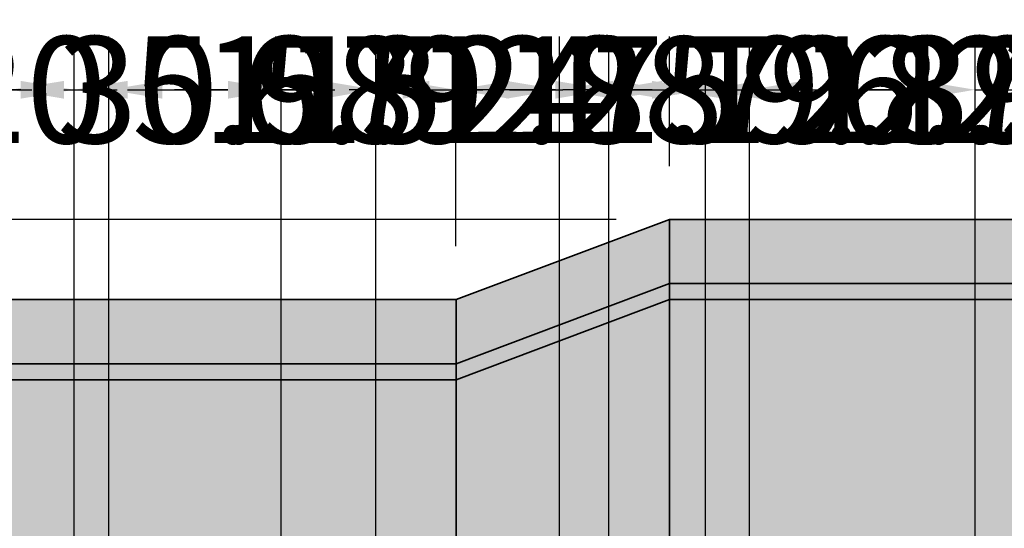
# Model space of a CAD drawing. Units: millimetres. Extents: x 130 to 1021, y 147 to 699.
# Tile 35 of 40: x 366 to 550, y 604 to 699. Entities that reach past the tile are written whole.
import ezdxf

# ---------------------------------------------------------------- set-up
doc = ezdxf.new("R2010")
doc.units = ezdxf.units.MM
doc.header["$MEASUREMENT"] = 0
for name, color, linetype, lineweight in [('A-ANNO-DIMS', 2, 'Continuous', 18), ('A-ELEV', 7, 'Continuous', 35), ('A-ELEV-PATT', 9, 'Continuous', 13)]:
    doc.layers.add(name, color=color, linetype=linetype, lineweight=lineweight)
doc.styles.get("Standard").update_dxf_attribs({"font": 'arial.ttf'})
doc.dimstyles.get("Standard").update_dxf_attribs({"dimtxt": 20, "dimasz": 10, "dimexe": 10, "dimexo": 10, "dimgap": 5, "dimtad": 0, "dimtih": 1, "dimtoh": 1, "dimdec": 0, "dimzin": 0, "dimdsep": 46, "dimtxsty": 'Standard', "dimcen": 5, "dimadec": 0, "dimazin": 0, "dimtfac": 1, "dimtdec": 0, "dimtofl": 0, "dimtmove": 0, "dimatfit": 3, "dimfxl": 1, "dimtolj": 1, "dimtzin": 0, "dimarcsym": 0})

# ---------------------------------------------------------------- blocks, each defined once
blk = doc.blocks.new('*D11')
at = {"layer": 'A-ANNO-DIMS', "color": 0, "lineweight": -2, "transparency": 16777216}
for p, q in [((737.37, 648.7), (737.37, 149.74)), ((299.37, 566.95), (299.37, 149.74)), ((309.37, 159.74), (490.86, 159.74)), ((727.37, 159.74), (545.89, 159.74))]:
    blk.add_line(p, q, dxfattribs=at)
at = {"layer": 'A-ANNO-DIMS', "color": 0, "transparency": 16777216}
for points in [[(309.37, 161.41), (309.37, 158.07), (299.37, 159.74)], [(727.37, 161.41), (727.37, 158.07), (737.37, 159.74)]]:
    blk.add_solid(points, dxfattribs=at)
at = {"layer": 'Defpoints', "color": 0, "transparency": 16777216}
for p in [(737.37, 658.7), (299.37, 576.95), (737.37, 159.74)]:
    blk.add_point(p, dxfattribs=at)
at = {"layer": 'A-ANNO-DIMS', "color": 0, "transparency": 16777216, "insert": (518.37, 159.74), "char_height": 20, "attachment_point": 5}
blk.add_mtext('\\A1;438', dxfattribs=at)
blk = doc.blocks.new('*D12')
at = {"layer": 'A-ANNO-DIMS', "color": 0, "lineweight": -2, "transparency": 16777216}
for p, q in [((477.37, 661.95), (265.07, 661.95)), ((275.07, 651.95), (275.07, 438.2)), ((275.07, 194.04), (275.07, 407.78)), ((357.16, 184.04), (265.07, 184.04))]:
    blk.add_line(p, q, dxfattribs=at)
at = {"layer": 'A-ANNO-DIMS', "color": 0, "transparency": 16777216}
for points in [[(273.41, 651.95), (276.74, 651.95), (275.07, 661.95)], [(273.41, 194.04), (276.74, 194.04), (275.07, 184.04)]]:
    blk.add_solid(points, dxfattribs=at)
at = {"layer": 'Defpoints', "color": 0, "transparency": 16777216}
for p in [(275.07, 661.95), (487.37, 661.95), (367.16, 184.04)]:
    blk.add_point(p, dxfattribs=at)
at = {"layer": 'A-ANNO-DIMS', "color": 0, "transparency": 16777216, "insert": (275.07, 422.99), "char_height": 20, "attachment_point": 5}
blk.add_mtext('\\A1;477.9', dxfattribs=at)
blk = doc.blocks.new('*D14')
at = {"layer": 'A-ANNO-DIMS', "color": 0, "lineweight": -2, "transparency": 16777216}
for p, q in [((307.37, 641.95), (307.37, 696.25)), ((327.37, 579.88), (327.37, 696.25)), ((297.37, 686.25), (287.37, 686.25)), ((337.37, 686.25), (347.37, 686.25))]:
    blk.add_line(p, q, dxfattribs=at)
at = {"layer": 'A-ANNO-DIMS', "color": 0, "transparency": 16777216}
for points in [[(297.37, 687.91), (297.37, 684.58), (307.37, 686.25)], [(337.37, 687.91), (337.37, 684.58), (327.37, 686.25)]]:
    blk.add_solid(points, dxfattribs=at)
at = {"layer": 'Defpoints', "color": 0, "transparency": 16777216}
for p in [(327.37, 686.25), (307.37, 631.95), (327.37, 569.88)]:
    blk.add_point(p, dxfattribs=at)
at = {"layer": 'A-ANNO-DIMS', "color": 0, "transparency": 16777216, "insert": (366.83, 686.25), "char_height": 20, "attachment_point": 5}
blk.add_mtext('\\A1;20', dxfattribs=at)
blk = doc.blocks.new('*D15')
at = {"layer": 'A-ANNO-DIMS', "color": 0, "lineweight": -2, "transparency": 16777216}
for p, q in [((327.37, 579.88), (327.37, 696.25)), ((357.94, 411.95), (357.94, 696.25)), ((337.37, 686.25), (347.94, 686.25)), ((357.94, 686.25), (367.94, 686.25))]:
    blk.add_line(p, q, dxfattribs=at)
at = {"layer": 'A-ANNO-DIMS', "color": 0, "transparency": 16777216}
for points in [[(337.37, 687.91), (337.37, 684.58), (327.37, 686.25)], [(347.94, 687.91), (347.94, 684.58), (357.94, 686.25)]]:
    blk.add_solid(points, dxfattribs=at)
at = {"layer": 'Defpoints', "color": 0, "transparency": 16777216}
for p in [(357.94, 686.25), (327.37, 569.88), (357.94, 401.95)]:
    blk.add_point(p, dxfattribs=at)
at = {"layer": 'A-ANNO-DIMS', "color": 0, "transparency": 16777216, "insert": (406.68, 686.25), "char_height": 20, "attachment_point": 5}
blk.add_mtext('\\A1;30.57', dxfattribs=at)
blk = doc.blocks.new('*D16')
at = {"layer": 'A-ANNO-DIMS', "color": 0, "lineweight": -2, "transparency": 16777216}
for p, q in [((357.94, 411.95), (357.94, 696.25)), ((363.92, 579.88), (363.92, 696.25)), ((347.94, 686.25), (337.94, 686.25)), ((373.92, 686.25), (383.92, 686.25))]:
    blk.add_line(p, q, dxfattribs=at)
at = {"layer": 'A-ANNO-DIMS', "color": 0, "transparency": 16777216}
for points in [[(347.94, 687.91), (347.94, 684.58), (357.94, 686.25)], [(373.92, 687.91), (373.92, 684.58), (363.92, 686.25)]]:
    blk.add_solid(points, dxfattribs=at)
at = {"layer": 'Defpoints', "color": 0, "transparency": 16777216}
for p in [(363.92, 686.25), (363.92, 569.88), (357.94, 401.95)]:
    blk.add_point(p, dxfattribs=at)
at = {"layer": 'A-ANNO-DIMS', "color": 0, "transparency": 16777216, "insert": (420.74, 686.25), "char_height": 20, "attachment_point": 5}
blk.add_mtext('\\A1;5.981', dxfattribs=at)
blk = doc.blocks.new('*D17')
at = {"layer": 'A-ANNO-DIMS', "color": 0, "lineweight": -2, "transparency": 16777216}
for p, q in [((363.92, 579.88), (363.92, 696.25)), ((375.85, 490.22), (375.85, 696.25)), ((353.92, 686.25), (343.92, 686.25)), ((385.85, 686.25), (395.85, 686.25))]:
    blk.add_line(p, q, dxfattribs=at)
at = {"layer": 'A-ANNO-DIMS', "color": 0, "transparency": 16777216}
for points in [[(353.92, 687.91), (353.92, 684.58), (363.92, 686.25)], [(385.85, 687.91), (385.85, 684.58), (375.85, 686.25)]]:
    blk.add_solid(points, dxfattribs=at)
at = {"layer": 'Defpoints', "color": 0, "transparency": 16777216}
for p in [(375.85, 686.25), (363.92, 569.88), (375.85, 480.22)]:
    blk.add_point(p, dxfattribs=at)
at = {"layer": 'A-ANNO-DIMS', "color": 0, "transparency": 16777216, "insert": (441.44, 686.25), "char_height": 20, "attachment_point": 5}
blk.add_mtext('\\A1;11.928', dxfattribs=at)
blk = doc.blocks.new('*D18')
at = {"layer": 'A-ANNO-DIMS', "color": 0, "lineweight": -2, "transparency": 16777216}
for p, q in [((375.85, 490.22), (375.85, 696.25)), ((382.37, 388.95), (382.37, 696.25)), ((365.85, 686.25), (355.85, 686.25)), ((392.37, 686.25), (402.37, 686.25))]:
    blk.add_line(p, q, dxfattribs=at)
at = {"layer": 'A-ANNO-DIMS', "color": 0, "transparency": 16777216}
for points in [[(365.85, 687.91), (365.85, 684.58), (375.85, 686.25)], [(392.37, 687.91), (392.37, 684.58), (382.37, 686.25)]]:
    blk.add_solid(points, dxfattribs=at)
at = {"layer": 'Defpoints', "color": 0, "transparency": 16777216}
for p in [(382.37, 686.25), (375.85, 480.22), (382.37, 378.95)]:
    blk.add_point(p, dxfattribs=at)
at = {"layer": 'A-ANNO-DIMS', "color": 0, "transparency": 16777216, "insert": (441.13, 686.25), "char_height": 20, "attachment_point": 5}
blk.add_mtext('\\A1;6.524', dxfattribs=at)
blk = doc.blocks.new('*D19')
at = {"layer": 'A-ANNO-DIMS', "color": 0, "lineweight": -2, "transparency": 16777216}
for p, q in [((382.37, 388.95), (382.37, 696.25)), ((414.65, 510.88), (414.65, 696.25)), ((392.37, 686.25), (404.65, 686.25)), ((414.65, 686.25), (424.65, 686.25))]:
    blk.add_line(p, q, dxfattribs=at)
at = {"layer": 'A-ANNO-DIMS', "color": 0, "transparency": 16777216}
for points in [[(392.37, 687.91), (392.37, 684.58), (382.37, 686.25)], [(404.65, 687.91), (404.65, 684.58), (414.65, 686.25)]]:
    blk.add_solid(points, dxfattribs=at)
at = {"layer": 'Defpoints', "color": 0, "transparency": 16777216}
for p in [(414.65, 686.25), (414.65, 500.88), (382.37, 378.95)]:
    blk.add_point(p, dxfattribs=at)
at = {"layer": 'A-ANNO-DIMS', "color": 0, "transparency": 16777216, "insert": (463.41, 686.25), "char_height": 20, "attachment_point": 5}
blk.add_mtext('\\A1;32.28', dxfattribs=at)
blk = doc.blocks.new('*D20')
at = {"layer": 'A-ANNO-DIMS', "color": 0, "lineweight": -2, "transparency": 16777216}
for p, q in [((414.65, 510.88), (414.65, 696.25)), ((432.37, 388.95), (432.37, 696.25)), ((404.65, 686.25), (394.65, 686.25)), ((442.37, 686.25), (452.37, 686.25))]:
    blk.add_line(p, q, dxfattribs=at)
at = {"layer": 'A-ANNO-DIMS', "color": 0, "transparency": 16777216}
for points in [[(404.65, 687.91), (404.65, 684.58), (414.65, 686.25)], [(442.37, 687.91), (442.37, 684.58), (432.37, 686.25)]]:
    blk.add_solid(points, dxfattribs=at)
at = {"layer": 'Defpoints', "color": 0, "transparency": 16777216}
for p in [(432.37, 686.25), (414.65, 500.88), (432.37, 378.95)]:
    blk.add_point(p, dxfattribs=at)
at = {"layer": 'A-ANNO-DIMS', "color": 0, "transparency": 16777216, "insert": (490.08, 686.25), "char_height": 20, "attachment_point": 5}
blk.add_mtext('\\A1;17.72', dxfattribs=at)
blk = doc.blocks.new('*D21')
at = {"layer": 'A-ANNO-DIMS', "color": 0, "lineweight": -2, "transparency": 16777216}
for p, q in [((432.37, 388.95), (432.37, 696.25)), ((447.37, 656.95), (447.37, 696.25)), ((422.37, 686.25), (412.37, 686.25)), ((457.37, 686.25), (467.37, 686.25))]:
    blk.add_line(p, q, dxfattribs=at)
at = {"layer": 'A-ANNO-DIMS', "color": 0, "transparency": 16777216}
for points in [[(422.37, 687.91), (422.37, 684.58), (432.37, 686.25)], [(457.37, 687.91), (457.37, 684.58), (447.37, 686.25)]]:
    blk.add_solid(points, dxfattribs=at)
at = {"layer": 'Defpoints', "color": 0, "transparency": 16777216}
for p in [(447.37, 686.25), (447.37, 646.95), (432.37, 378.95)]:
    blk.add_point(p, dxfattribs=at)
at = {"layer": 'A-ANNO-DIMS', "color": 0, "transparency": 16777216, "insert": (485.83, 686.25), "char_height": 20, "attachment_point": 5}
blk.add_mtext('\\A1;15', dxfattribs=at)
blk = doc.blocks.new('*D22')
at = {"layer": 'A-ANNO-DIMS', "color": 0, "lineweight": -2, "transparency": 16777216}
for p, q in [((447.37, 656.95), (447.37, 696.25)), ((466.77, 403.95), (466.77, 696.25)), ((437.37, 686.25), (427.37, 686.25)), ((476.77, 686.25), (486.77, 686.25))]:
    blk.add_line(p, q, dxfattribs=at)
at = {"layer": 'A-ANNO-DIMS', "color": 0, "transparency": 16777216}
for points in [[(437.37, 687.91), (437.37, 684.58), (447.37, 686.25)], [(476.77, 687.91), (476.77, 684.58), (466.77, 686.25)]]:
    blk.add_solid(points, dxfattribs=at)
at = {"layer": 'Defpoints', "color": 0, "transparency": 16777216}
for p in [(466.77, 686.25), (447.37, 646.95), (466.77, 393.95)]:
    blk.add_point(p, dxfattribs=at)
at = {"layer": 'A-ANNO-DIMS', "color": 0, "transparency": 16777216, "insert": (532.34, 686.25), "char_height": 20, "attachment_point": 5}
blk.add_mtext('\\A1;19.393', dxfattribs=at)
blk = doc.blocks.new('*D23')
at = {"layer": 'A-ANNO-DIMS', "color": 0, "lineweight": -2, "transparency": 16777216}
for p, q in [((466.77, 403.95), (466.77, 696.25)), ((475.99, 209.04), (475.99, 696.25)), ((456.77, 686.25), (446.77, 686.25)), ((485.99, 686.25), (495.99, 686.25))]:
    blk.add_line(p, q, dxfattribs=at)
at = {"layer": 'A-ANNO-DIMS', "color": 0, "transparency": 16777216}
for points in [[(456.77, 687.91), (456.77, 684.58), (466.77, 686.25)], [(485.99, 687.91), (485.99, 684.58), (475.99, 686.25)]]:
    blk.add_solid(points, dxfattribs=at)
at = {"layer": 'Defpoints', "color": 0, "transparency": 16777216}
for p in [(475.99, 686.25), (466.77, 393.95), (475.99, 199.04)]:
    blk.add_point(p, dxfattribs=at)
at = {"layer": 'A-ANNO-DIMS', "color": 0, "transparency": 16777216, "insert": (534.63, 686.25), "char_height": 20, "attachment_point": 5}
blk.add_mtext('\\A1;9.222', dxfattribs=at)
blk = doc.blocks.new('*D24')
at = {"layer": 'A-ANNO-DIMS', "color": 0, "lineweight": -2, "transparency": 16777216}
for p, q in [((475.99, 209.04), (475.99, 696.25)), ((487.37, 671.95), (487.37, 696.25)), ((465.99, 686.25), (455.99, 686.25)), ((497.37, 686.25), (507.37, 686.25))]:
    blk.add_line(p, q, dxfattribs=at)
at = {"layer": 'A-ANNO-DIMS', "color": 0, "transparency": 16777216}
for points in [[(465.99, 687.91), (465.99, 684.58), (475.99, 686.25)], [(497.37, 687.91), (497.37, 684.58), (487.37, 686.25)]]:
    blk.add_solid(points, dxfattribs=at)
at = {"layer": 'Defpoints', "color": 0, "transparency": 16777216}
for p in [(487.37, 686.25), (487.37, 661.95), (475.99, 199.04)]:
    blk.add_point(p, dxfattribs=at)
at = {"layer": 'A-ANNO-DIMS', "color": 0, "transparency": 16777216, "insert": (553.02, 686.25), "char_height": 20, "attachment_point": 5}
blk.add_mtext('\\A1;11.385', dxfattribs=at)
blk = doc.blocks.new('*D25')
at = {"layer": 'A-ANNO-DIMS', "color": 0, "lineweight": -2, "transparency": 16777216}
for p, q in [((487.37, 671.95), (487.37, 696.25)), ((494.1, 506.91), (494.1, 696.25)), ((477.37, 686.25), (467.37, 686.25)), ((504.1, 686.25), (514.1, 686.25))]:
    blk.add_line(p, q, dxfattribs=at)
at = {"layer": 'A-ANNO-DIMS', "color": 0, "transparency": 16777216}
for points in [[(477.37, 687.91), (477.37, 684.58), (487.37, 686.25)], [(504.1, 687.91), (504.1, 684.58), (494.1, 686.25)]]:
    blk.add_solid(points, dxfattribs=at)
at = {"layer": 'Defpoints', "color": 0, "transparency": 16777216}
for p in [(494.1, 686.25), (487.37, 661.95), (494.1, 496.91)]:
    blk.add_point(p, dxfattribs=at)
at = {"layer": 'A-ANNO-DIMS', "color": 0, "transparency": 16777216, "insert": (552.92, 686.25), "char_height": 20, "attachment_point": 5}
blk.add_mtext('\\A1;6.728', dxfattribs=at)
blk = doc.blocks.new('*D26')
at = {"layer": 'A-ANNO-DIMS', "color": 0, "lineweight": -2, "transparency": 16777216}
for p, q in [((494.1, 506.91), (494.1, 696.25)), ((502.37, 593.95), (502.37, 696.25)), ((484.1, 686.25), (474.1, 686.25)), ((512.37, 686.25), (522.37, 686.25))]:
    blk.add_line(p, q, dxfattribs=at)
at = {"layer": 'A-ANNO-DIMS', "color": 0, "transparency": 16777216}
for points in [[(484.1, 687.91), (484.1, 684.58), (494.1, 686.25)], [(512.37, 687.91), (512.37, 684.58), (502.37, 686.25)]]:
    blk.add_solid(points, dxfattribs=at)
at = {"layer": 'Defpoints', "color": 0, "transparency": 16777216}
for p in [(502.37, 686.25), (502.37, 583.95), (494.1, 496.91)]:
    blk.add_point(p, dxfattribs=at)
at = {"layer": 'A-ANNO-DIMS', "color": 0, "transparency": 16777216, "insert": (561.03, 686.25), "char_height": 20, "attachment_point": 5}
blk.add_mtext('\\A1;8.272', dxfattribs=at)
blk = doc.blocks.new('*D27')
at = {"layer": 'A-ANNO-DIMS', "color": 0, "lineweight": -2, "transparency": 16777216}
for p, q in [((502.37, 593.95), (502.37, 696.25)), ((544.64, 396.26), (544.64, 696.25)), ((512.37, 686.25), (534.64, 686.25)), ((544.64, 686.25), (554.64, 686.25))]:
    blk.add_line(p, q, dxfattribs=at)
at = {"layer": 'A-ANNO-DIMS', "color": 0, "transparency": 16777216}
for points in [[(512.37, 687.91), (512.37, 684.58), (502.37, 686.25)], [(534.64, 687.91), (534.64, 684.58), (544.64, 686.25)]]:
    blk.add_solid(points, dxfattribs=at)
at = {"layer": 'Defpoints', "color": 0, "transparency": 16777216}
for p in [(544.64, 686.25), (502.37, 583.95), (544.64, 386.26)]:
    blk.add_point(p, dxfattribs=at)
at = {"layer": 'A-ANNO-DIMS', "color": 0, "transparency": 16777216, "insert": (593.78, 686.25), "char_height": 20, "attachment_point": 5}
blk.add_mtext('\\A1;42.26', dxfattribs=at)
blk = doc.blocks.new('*D28')
at = {"layer": 'A-ANNO-DIMS', "color": 0, "lineweight": -2, "transparency": 16777216}
for p, q in [((544.64, 396.26), (544.64, 696.25)), ((552.37, 593.95), (552.37, 696.25)), ((534.64, 686.25), (524.64, 686.25)), ((562.37, 686.25), (572.37, 686.25))]:
    blk.add_line(p, q, dxfattribs=at)
at = {"layer": 'A-ANNO-DIMS', "color": 0, "transparency": 16777216}
for points in [[(534.64, 687.91), (534.64, 684.58), (544.64, 686.25)], [(562.37, 687.91), (562.37, 684.58), (552.37, 686.25)]]:
    blk.add_solid(points, dxfattribs=at)
at = {"layer": 'Defpoints', "color": 0, "transparency": 16777216}
for p in [(552.37, 686.25), (552.37, 583.95), (544.64, 386.26)]:
    blk.add_point(p, dxfattribs=at)
at = {"layer": 'A-ANNO-DIMS', "color": 0, "transparency": 16777216, "insert": (611.06, 686.25), "char_height": 20, "attachment_point": 5}
blk.add_mtext('\\A1;7.738', dxfattribs=at)
blk = doc.blocks.new('*D57')
at = {"layer": 'A-ANNO-DIMS', "color": 0, "lineweight": -2, "transparency": 16777216}
for p, q in [((761.67, 606.95), (761.67, 616.95)), ((761.67, 616.95), (771.67, 616.95)), ((497.37, 596.95), (771.67, 596.95)), ((562.37, 583.95), (771.67, 583.95)), ((761.67, 573.95), (761.67, 563.95))]:
    blk.add_line(p, q, dxfattribs=at)
at = {"layer": 'A-ANNO-DIMS', "color": 0, "transparency": 16777216}
for points in [[(760.01, 606.95), (763.34, 606.95), (761.67, 596.95)], [(760.01, 573.95), (763.34, 573.95), (761.67, 583.95)]]:
    blk.add_solid(points, dxfattribs=at)
at = {"layer": 'Defpoints', "color": 0, "transparency": 16777216}
for p in [(487.37, 596.95), (761.67, 596.95), (552.37, 583.95)]:
    blk.add_point(p, dxfattribs=at)
at = {"layer": 'A-ANNO-DIMS', "color": 0, "transparency": 16777216, "insert": (790.06, 616.95), "char_height": 20, "attachment_point": 5}
blk.add_mtext('\\A1;13', dxfattribs=at)
blk = doc.blocks.new('*D58')
at = {"layer": 'A-ANNO-DIMS', "color": 0, "lineweight": -2, "transparency": 16777216}
for p, q in [((761.67, 656.95), (761.67, 666.95)), ((497.37, 646.95), (771.67, 646.95)), ((497.37, 596.95), (771.67, 596.95)), ((761.67, 586.95), (761.67, 576.95))]:
    blk.add_line(p, q, dxfattribs=at)
at = {"layer": 'A-ANNO-DIMS', "color": 0, "transparency": 16777216}
for points in [[(760.01, 656.95), (763.34, 656.95), (761.67, 646.95)], [(760.01, 586.95), (763.34, 586.95), (761.67, 596.95)]]:
    blk.add_solid(points, dxfattribs=at)
at = {"layer": 'Defpoints', "color": 0, "transparency": 16777216}
for p in [(487.37, 646.95), (761.67, 646.95), (487.37, 596.95)]:
    blk.add_point(p, dxfattribs=at)
at = {"layer": 'A-ANNO-DIMS', "color": 0, "transparency": 16777216, "insert": (761.67, 621.95), "char_height": 20, "attachment_point": 5}
blk.add_mtext('\\A1;50', dxfattribs=at)
blk = doc.blocks.new('*D59')
at = {"layer": 'A-ANNO-DIMS', "color": 0, "lineweight": -2, "transparency": 16777216}
for p, q in [((761.67, 671.95), (761.67, 681.95)), ((761.67, 681.95), (771.67, 681.95)), ((497.37, 661.95), (771.67, 661.95)), ((497.37, 646.95), (771.67, 646.95)), ((761.67, 636.95), (761.67, 626.95))]:
    blk.add_line(p, q, dxfattribs=at)
at = {"layer": 'A-ANNO-DIMS', "color": 0, "transparency": 16777216}
for points in [[(760.01, 671.95), (763.34, 671.95), (761.67, 661.95)], [(760.01, 636.95), (763.34, 636.95), (761.67, 646.95)]]:
    blk.add_solid(points, dxfattribs=at)
at = {"layer": 'Defpoints', "color": 0, "transparency": 16777216}
for p in [(487.37, 661.95), (761.67, 661.95), (487.37, 646.95)]:
    blk.add_point(p, dxfattribs=at)
at = {"layer": 'A-ANNO-DIMS', "color": 0, "transparency": 16777216, "insert": (790.13, 681.95), "char_height": 20, "attachment_point": 5}
blk.add_mtext('\\A1;15', dxfattribs=at)

msp = doc.modelspace()

# ---------------------------------------------------------------- hatches: boundary and pattern name
at = {"layer": 'A-ELEV-PATT'}
h = msp.add_hatch(color=256, dxfattribs=at)
h.dxf.hatch_style = 1
h.paths.add_polyline_path([(737.3738, 658.6988, 0.01359606), (632.4019, 661.9473), (607.3738, 661.9473), (487.3738, 661.9473), (487.3738, 649.9473), (607.3738, 649.9473), (632.3794, 649.9473, -0.01368411), (737.3738, 646.6784)])
h.paths.add_polyline_path([(732.3738, 643.9599, 0.01305286), (632.3738, 646.9473), (607.3738, 646.9473), (487.3738, 646.9473), (487.3738, 596.9473), (632.3738, 596.9473, -0.01305286), (732.3738, 593.9599)])
h.paths.add_polyline_path([(737.3738, 593.6732, 0.01370629), (632.3738, 596.9473), (487.3738, 596.9473), (487.3738, 586.9473), (632.355, 586.9473, -0.01378075), (737.3738, 583.6559)])
h.paths.add_polyline_path([(447.3738, 646.9473), (307.3738, 646.9473), (302.3738, 646.9473), (302.3738, 634.9473), (447.3738, 634.9473)])
h.paths.add_polyline_path([(447.3738, 631.9473), (307.3738, 631.9473), (307.3738, 586.9473), (447.3738, 586.9473)])
h.paths.add_polyline_path([(447.3738, 586.9473), (307.3738, 586.9473), (302.3738, 586.9473), (302.3738, 576.9473), (447.3738, 576.9473)])
h.paths.add_polyline_path([(447.3738, 573.9473), (367.3738, 573.9473), (367.3738, 539.9473), (447.3738, 539.9473)])
h.paths.add_polyline_path([(447.3738, 537.9473), (367.3738, 537.9473), (367.3738, 507.9473), (400.392, 507.4253, -0.00172798), (401.3281, 507.6451, -0.52200255), (425.6117, 511.0391, -0.03918489), (447.3738, 510.4359), (447.3738, 510.7883)])
h.paths.add_polyline_path([(394.7238, 505.9473), (367.3738, 505.9473), (367.3738, 476.9473, -0.0146512), (375.8501, 480.2159), (376.1506, 499.2266, -0.03554194)])
h.paths.add_polyline_path([(632.3738, 583.9473), (552.3738, 583.9473), (552.3738, 550.9473), (632.3738, 550.9473)])
h.paths.add_polyline_path([(632.3738, 548.9473), (552.3738, 548.9473), (552.3738, 515.9473), (632.3738, 515.9473)])
h.paths.add_polyline_path([(632.3738, 513.9473), (552.3738, 513.9473), (552.3738, 476.9473), (632.3738, 476.9473)])
h.paths.add_polyline_path([(737.3738, 473.6903, 0.01363261), (632.3926, 476.9473), (552.3738, 476.9473), (487.3738, 476.9473), (487.3738, 466.9473), (632.3738, 466.9473, -0.01370629), (737.3738, 463.6732)])
h.paths.add_polyline_path([(732.3738, 460.9552, 0.01307409), (632.3681, 463.9473), (487.3738, 463.9473), (487.3738, 407.735, -0.00322862), (489.3544, 406.9473), (632.3926, 406.9473, -0.01298259), (732.3738, 403.9755)])
h.paths.add_polyline_path([(487.3738, 463.9473, 0.20132998), (367.3738, 463.9473), (367.3738, 407.735, -0.18820307), (487.3738, 407.735)])
h.paths.add_polyline_path([(367.3738, 476.9473), (367.3738, 466.9473, -0.20133085), (487.3738, 466.9473), (487.3738, 476.9473, 0.20132998)])
h.paths.add_polyline_path([(367.3738, 463.9473), (307.3738, 463.9473), (307.3738, 401.9473), (357.9413, 401.9473), (367.3738, 407.735)])
h.paths.add_polyline_path([(367.3738, 476.9473), (302.3738, 476.9473), (302.3738, 466.9473), (367.3738, 466.9473)])
h.paths.add_polyline_path([(632.8184, 366.9453), (552.3738, 366.9453), (552.3738, 393.9473), (632.8184, 393.9473)])
h.paths.add_polyline_path([(632.8184, 357.2114), (632.8184, 363.9453), (552.3738, 363.9453), (552.3738, 357.2114), (552.3738, 336.9453), (632.8184, 336.9453)])
h.paths.add_polyline_path([(632.8184, 333.9453), (552.3738, 333.9453), (552.3738, 306.9453), (632.8184, 306.9453)])
h.paths.add_polyline_path([(632.8184, 303.9453), (552.3738, 303.9453), (552.3738, 273.9473), (632.355, 273.9473, 0.00006077), (632.8184, 273.9491)])
h.paths.add_polyline_path([(737.3738, 403.6903, 0.01363261), (632.3926, 406.9473), (489.3544, 406.9473, 0.19154808), (367.3738, 407.735), (367.3738, 396.9473, -0.20133085), (487.3738, 396.9473), (632.3738, 396.9473, -0.01370629), (737.3738, 393.6732)])
h.paths.add_polyline_path([(357.9413, 401.9473), (307.3738, 401.9473), (307.3738, 391.9473), (357.9413, 391.9473)])
h.paths.add_polyline_path([(357.9413, 357.2114), (357.9413, 388.9473), (307.3738, 388.9473), (307.3738, 357.2114), (307.3738, 273.9473), (357.9413, 273.9473)])
h.paths.add_polyline_path([(732.3738, 263.93, -0.0130317), (632.3794, 260.9473), (466.7667, 260.9473), (466.7667, 240.9473), (469.8406, 236.978), (469.8406, 221.978), (472.9145, 218.0087), (472.9145, 213.9473), (607.3738, 213.9473), (732.3738, 213.9473)])
h.paths.add_polyline_path([(732.3738, 290.889), (722.479, 290.889), (722.479, 301.889), (732.3738, 301.889), (732.3738, 305.889), (722.479, 305.889), (722.479, 316.889), (732.3738, 316.889), (732.3738, 320.889), (722.479, 320.889), (722.479, 331.889), (732.3738, 331.889), (732.3738, 335.889), (722.479, 335.889), (722.479, 346.889), (732.3738, 346.889), (732.3738, 350.889), (722.479, 350.889), (722.479, 361.889), (732.3738, 361.889), (732.3738, 365.889), (722.479, 365.889), (722.479, 376.889), (732.3738, 376.889), (732.3738, 380.889), (722.479, 380.889), (722.479, 391.4848, 0.00052326), (718.479, 391.6843), (718.479, 380.889), (707.479, 380.889), (707.479, 392.1896, 0.00052307), (703.479, 392.3576), (703.479, 380.889), (692.479, 380.889), (692.479, 392.7765, 0.00052292), (688.479, 392.9131), (688.479, 380.889), (677.479, 380.889), (677.479, 393.2456, 0.00052279), (673.479, 393.3508), (673.479, 380.889), (662.479, 380.889), (662.479, 393.597, 0.0005227), (658.479, 393.6709), (658.479, 380.889), (647.479, 380.889), (647.479, 393.8308, 0.00052264), (643.479, 393.8732), (643.479, 380.889), (632.8184, 380.889), (632.8184, 376.889), (643.479, 376.889), (643.479, 365.889), (632.8184, 365.889), (632.8184, 361.889), (643.479, 361.889), (643.479, 350.889), (632.8184, 350.889), (632.8184, 346.889), (643.479, 346.889), (643.479, 335.889), (632.8184, 335.889), (632.8184, 331.889), (643.479, 331.889), (643.479, 320.889), (632.8184, 320.889), (632.8184, 316.889), (643.479, 316.889), (643.479, 305.889), (632.8184, 305.889), (632.8184, 301.889), (643.479, 301.889), (643.479, 290.889), (632.8184, 290.889), (632.8184, 286.889), (643.479, 286.889), (643.479, 274.0217, 0.00052456), (647.479, 274.0643), (647.479, 286.889), (658.479, 286.889), (658.479, 274.2248, 0.00052462), (662.479, 274.2989), (662.479, 286.889), (673.479, 286.889), (673.479, 274.546, 0.00052471), (677.479, 274.6516), (677.479, 286.889), (688.479, 286.889), (688.479, 274.9853, 0.00052484), (692.479, 275.1224), (692.479, 286.889), (703.479, 286.889), (703.479, 275.5429, 0.000525), (707.479, 275.7115), (707.479, 286.889), (718.479, 286.889), (718.479, 276.2187, 0.00052519), (722.479, 276.4189), (722.479, 286.889), (732.3738, 286.889)])
h.paths.add_polyline_path([(718.479, 290.889), (707.479, 290.889), (707.479, 301.889), (718.479, 301.889)], flags=16)
h.paths.add_polyline_path([(703.479, 290.889), (692.479, 290.889), (692.479, 301.889), (703.479, 301.889)], flags=16)
h.paths.add_polyline_path([(718.479, 305.889), (707.479, 305.889), (707.479, 316.889), (718.479, 316.889)], flags=16)
h.paths.add_polyline_path([(703.479, 305.889), (692.479, 305.889), (692.479, 316.889), (703.479, 316.889)], flags=16)
h.paths.add_polyline_path([(688.479, 290.889), (677.479, 290.889), (677.479, 301.889), (688.479, 301.889)], flags=16)
h.paths.add_polyline_path([(718.479, 320.889), (707.479, 320.889), (707.479, 331.889), (718.479, 331.889)], flags=16)
h.paths.add_polyline_path([(688.479, 305.889), (677.479, 305.889), (677.479, 316.889), (688.479, 316.889)], flags=16)
h.paths.add_polyline_path([(703.479, 320.889), (692.479, 320.889), (692.479, 331.889), (703.479, 331.889)], flags=16)
h.paths.add_polyline_path([(688.479, 320.889), (677.479, 320.889), (677.479, 331.889), (688.479, 331.889)], flags=16)
h.paths.add_polyline_path([(673.479, 290.889), (662.479, 290.889), (662.479, 301.889), (673.479, 301.889)], flags=16)
h.paths.add_polyline_path([(718.479, 335.889), (707.479, 335.889), (707.479, 346.889), (718.479, 346.889)], flags=16)
h.paths.add_polyline_path([(673.479, 305.889), (662.479, 305.889), (662.479, 316.889), (673.479, 316.889)], flags=16)
h.paths.add_polyline_path([(703.479, 335.889), (692.479, 335.889), (692.479, 346.889), (703.479, 346.889)], flags=16)
h.paths.add_polyline_path([(673.479, 320.889), (662.479, 320.889), (662.479, 331.889), (673.479, 331.889)], flags=16)
h.paths.add_polyline_path([(688.479, 335.889), (677.479, 335.889), (677.479, 346.889), (688.479, 346.889)], flags=16)
h.paths.add_polyline_path([(658.479, 290.889), (647.479, 290.889), (647.479, 301.889), (658.479, 301.889)], flags=16)
h.paths.add_polyline_path([(718.479, 350.889), (707.479, 350.889), (707.479, 361.889), (718.479, 361.889)], flags=16)
h.paths.add_polyline_path([(658.479, 305.889), (647.479, 305.889), (647.479, 316.889), (658.479, 316.889)], flags=16)
h.paths.add_polyline_path([(703.479, 350.889), (692.479, 350.889), (692.479, 361.889), (703.479, 361.889)], flags=16)
h.paths.add_polyline_path([(673.479, 335.889), (662.479, 335.889), (662.479, 346.889), (673.479, 346.889)], flags=16)
h.paths.add_polyline_path([(658.479, 320.889), (647.479, 320.889), (647.479, 331.889), (658.479, 331.889)], flags=16)
h.paths.add_polyline_path([(688.479, 350.889), (677.479, 350.889), (677.479, 361.889), (688.479, 361.889)], flags=16)
h.paths.add_polyline_path([(718.479, 365.889), (707.479, 365.889), (707.479, 376.889), (718.479, 376.889)], flags=16)
h.paths.add_polyline_path([(658.479, 335.889), (647.479, 335.889), (647.479, 346.889), (658.479, 346.889)], flags=16)
h.paths.add_polyline_path([(673.479, 350.889), (662.479, 350.889), (662.479, 361.889), (673.479, 361.889)], flags=16)
h.paths.add_polyline_path([(703.479, 365.889), (692.479, 365.889), (692.479, 376.889), (703.479, 376.889)], flags=16)
h.paths.add_polyline_path([(688.479, 365.889), (677.479, 365.889), (677.479, 376.889), (688.479, 376.889)], flags=16)
h.paths.add_polyline_path([(658.479, 350.889), (647.479, 350.889), (647.479, 361.889), (658.479, 361.889)], flags=16)
h.paths.add_polyline_path([(673.479, 365.889), (662.479, 365.889), (662.479, 376.889), (673.479, 376.889)], flags=16)
h.paths.add_polyline_path([(658.479, 365.889), (647.479, 365.889), (647.479, 376.889), (658.479, 376.889)], flags=16)
h.paths.add_polyline_path([(732.3738, 503.9786), (722.3392, 503.9786), (722.3392, 514.9786), (732.3738, 514.9786), (732.3738, 518.9786), (722.3392, 518.9786), (722.3392, 529.9786), (732.3738, 529.9786), (732.3738, 533.9786), (722.3392, 533.9786), (722.3392, 544.9786), (732.3738, 544.9786), (732.3738, 546.9473), (732.3738, 548.9786), (722.3392, 548.9786), (722.3392, 559.9786), (732.3738, 559.9786), (732.3738, 563.9786), (722.3392, 563.9786), (722.3392, 574.9786), (732.3738, 574.9786), (732.3738, 578.9786), (722.3392, 578.9786), (722.3392, 581.4789, 0.00052601), (718.3392, 581.6791), (718.3392, 578.9786), (707.3392, 578.9786), (707.3392, 582.1863, 0.00052582), (703.3392, 582.355), (703.3392, 578.9786), (692.3392, 578.9786), (692.3392, 582.7752, 0.00052566), (688.3392, 582.9123), (688.3392, 578.9786), (677.3392, 578.9786), (677.3392, 583.2457, 0.00052554), (673.3392, 583.3512), (673.3392, 578.9786), (662.3392, 578.9786), (662.3392, 583.5978, 0.00052545), (658.3392, 583.6718), (658.3392, 578.9786), (647.3392, 578.9786), (647.3392, 583.8317, 0.00052539), (643.3392, 583.8741), (643.3392, 578.9786), (632.3738, 578.9786), (632.3738, 574.9786), (643.3392, 574.9786), (643.3392, 563.9786), (632.3738, 563.9786), (632.3738, 559.9786), (643.3392, 559.9786), (643.3392, 548.9786), (632.3738, 548.9786), (632.3738, 544.9786), (643.3392, 544.9786), (643.3392, 533.9786), (632.3738, 533.9786), (632.3738, 529.9786), (643.3392, 529.9786), (643.3392, 518.9786), (632.3738, 518.9786), (632.3738, 515.9473), (632.3738, 514.9786), (643.3392, 514.9786), (643.3392, 503.9786), (632.3738, 503.9786), (632.3738, 499.9786), (643.3392, 499.9786), (643.3392, 488.9786), (632.3738, 488.9786), (632.3738, 484.9786), (643.3392, 484.9786), (643.3392, 476.8751, -0.00051911), (647.3392, 476.8332), (647.3392, 484.9786), (658.3392, 484.9786), (658.3392, 476.6752, -0.00051917), (662.3392, 476.6022), (662.3392, 484.9786), (673.3392, 484.9786), (673.3392, 476.3585, -0.00051926), (677.3392, 476.2543), (677.3392, 484.9786), (688.3392, 484.9786), (688.3392, 475.9248, -0.00051938), (692.3392, 475.7894), (692.3392, 484.9786), (703.3392, 484.9786), (703.3392, 475.3741, -0.00051953), (707.3392, 475.2075), (707.3392, 484.9786), (718.3392, 484.9786), (718.3392, 474.7064, -0.00051972), (722.3392, 474.5086), (722.3392, 484.9786), (732.3738, 484.9786), (732.3738, 488.9786), (722.3392, 488.9786), (722.3392, 499.9786), (732.3738, 499.9786)])
h.paths.add_polyline_path([(718.3392, 503.9786), (707.3392, 503.9786), (707.3392, 514.9786), (718.3392, 514.9786)], flags=16)
h.paths.add_polyline_path([(718.3392, 499.9786), (718.3392, 488.9786), (707.3392, 488.9786), (707.3392, 499.9786)], flags=16)
h.paths.add_polyline_path([(718.3392, 518.9786), (707.3392, 518.9786), (707.3392, 529.9786), (718.3392, 529.9786)], flags=16)
h.paths.add_polyline_path([(703.3392, 503.9786), (692.3392, 503.9786), (692.3392, 514.9786), (703.3392, 514.9786)], flags=16)
h.paths.add_polyline_path([(703.3392, 499.9786), (703.3392, 488.9786), (692.3392, 488.9786), (692.3392, 499.9786)], flags=16)
h.paths.add_polyline_path([(703.3392, 518.9786), (692.3392, 518.9786), (692.3392, 529.9786), (703.3392, 529.9786)], flags=16)
h.paths.add_polyline_path([(718.3392, 533.9786), (707.3392, 533.9786), (707.3392, 544.9786), (718.3392, 544.9786)], flags=16)
h.paths.add_polyline_path([(688.3392, 503.9786), (677.3392, 503.9786), (677.3392, 514.9786), (688.3392, 514.9786)], flags=16)
h.paths.add_polyline_path([(688.3392, 499.9786), (688.3392, 488.9786), (677.3392, 488.9786), (677.3392, 499.9786)], flags=16)
h.paths.add_polyline_path([(703.3392, 533.9786), (692.3392, 533.9786), (692.3392, 544.9786), (703.3392, 544.9786)], flags=16)
h.paths.add_polyline_path([(688.3392, 518.9786), (677.3392, 518.9786), (677.3392, 529.9786), (688.3392, 529.9786)], flags=16)
h.paths.add_polyline_path([(688.3392, 533.9786), (677.3392, 533.9786), (677.3392, 544.9786), (688.3392, 544.9786)], flags=16)
h.paths.add_polyline_path([(718.3392, 548.9786), (707.3392, 548.9786), (707.3392, 559.9786), (718.3392, 559.9786)], flags=16)
h.paths.add_polyline_path([(673.3392, 503.9786), (662.3392, 503.9786), (662.3392, 514.9786), (673.3392, 514.9786)], flags=16)
h.paths.add_polyline_path([(673.3392, 499.9786), (673.3392, 488.9786), (662.3392, 488.9786), (662.3392, 499.9786)], flags=16)
h.paths.add_polyline_path([(703.3392, 548.9786), (692.3392, 548.9786), (692.3392, 559.9786), (703.3392, 559.9786)], flags=16)
h.paths.add_polyline_path([(673.3392, 518.9786), (662.3392, 518.9786), (662.3392, 529.9786), (673.3392, 529.9786)], flags=16)
h.paths.add_polyline_path([(688.3392, 548.9786), (677.3392, 548.9786), (677.3392, 559.9786), (688.3392, 559.9786)], flags=16)
h.paths.add_polyline_path([(673.3392, 533.9786), (662.3392, 533.9786), (662.3392, 544.9786), (673.3392, 544.9786)], flags=16)
h.paths.add_polyline_path([(718.3392, 563.9786), (707.3392, 563.9786), (707.3392, 574.9786), (718.3392, 574.9786)], flags=16)
h.paths.add_polyline_path([(658.3392, 503.9786), (647.3392, 503.9786), (647.3392, 514.9786), (658.3392, 514.9786)], flags=16)
h.paths.add_polyline_path([(658.3392, 499.9786), (658.3392, 488.9786), (647.3392, 488.9786), (647.3392, 499.9786)], flags=16)
h.paths.add_polyline_path([(703.3392, 563.9786), (692.3392, 563.9786), (692.3392, 574.9786), (703.3392, 574.9786)], flags=16)
h.paths.add_polyline_path([(658.3392, 518.9786), (647.3392, 518.9786), (647.3392, 529.9786), (658.3392, 529.9786)], flags=16)
h.paths.add_polyline_path([(673.3392, 548.9786), (662.3392, 548.9786), (662.3392, 559.9786), (673.3392, 559.9786)], flags=16)
h.paths.add_polyline_path([(688.3392, 563.9786), (677.3392, 563.9786), (677.3392, 574.9786), (688.3392, 574.9786)], flags=16)
h.paths.add_polyline_path([(658.3392, 533.9786), (647.3392, 533.9786), (647.3392, 544.9786), (658.3392, 544.9786)], flags=16)
h.paths.add_polyline_path([(673.3392, 563.9786), (662.3392, 563.9786), (662.3392, 574.9786), (673.3392, 574.9786)], flags=16)
h.paths.add_polyline_path([(658.3392, 548.9786), (647.3392, 548.9786), (647.3392, 559.9786), (658.3392, 559.9786)], flags=16)
h.paths.add_polyline_path([(658.3392, 563.9786), (647.3392, 563.9786), (647.3392, 574.9786), (658.3392, 574.9786)], flags=16)
h = msp.add_hatch(color=256, dxfattribs=at)
h.dxf.hatch_style = 1
h.paths.add_polyline_path([(487.3738, 649.9473), (487.3738, 661.9473), (447.3738, 646.9473), (447.3738, 634.9473)])
h.paths.add_polyline_path([(487.3738, 646.9473), (447.3738, 631.9473), (447.3738, 586.9473), (487.3738, 596.9473)])
h.paths.add_polyline_path([(487.3738, 596.9473), (447.3738, 586.9473), (447.3738, 576.9473), (487.3738, 586.9473)])
h.paths.add_polyline_path([(460.3738, 577.1973), (447.3738, 573.9473), (447.3738, 510.7883), (447.3738, 510.4359, -0.02365365), (460.3738, 508.4268), (460.3738, 509.3636)])
h.paths.add_polyline_path([(472.3738, 580.1973), (460.3738, 577.1973), (460.3738, 509.3636), (460.3738, 508.4268, -0.00551471), (463.3738, 507.7821), (463.3738, 508.8807), (463.3738, 572.7934), (469.3738, 574.2934), (469.3738, 507.7378), (469.3738, 506.2825, -0.00560751), (472.3738, 505.4251), (472.3738, 507.0765)])
h = msp.add_hatch(color=256, dxfattribs=at)
h.dxf.hatch_style = 1
h.paths.add_polyline_path([(447.3738, 634.9473), (302.3738, 634.9473), (302.3738, 631.9473), (307.3738, 631.9473), (447.3738, 631.9473)])
h.paths.add_polyline_path([(487.3738, 646.9473), (487.3738, 649.9473), (447.3738, 634.9473), (447.3738, 631.9473)])
h.paths.add_polyline_path([(632.3794, 649.9473), (607.3738, 649.9473), (487.3738, 649.9473), (487.3738, 646.9473), (607.3738, 646.9473), (632.3738, 646.9473, -0.01370629), (737.3738, 643.6732), (737.3738, 646.6784, 0.01368411)])

# ---------------------------------------------------------------- linework, layer by layer
at = {"layer": 'A-ELEV'}
for p, q in [((487.3738, 661.9473), (447.3738, 646.9473)), ((487.3738, 646.9473), (487.3738, 661.9473)), ((607.3738, 661.9473), (487.3738, 661.9473)), ((487.3738, 649.9473), (447.3738, 634.9473)), ((607.3738, 649.9473), (487.3738, 649.9473)), ((447.3738, 646.9473), (307.3738, 646.9473)), ((447.3738, 646.9473), (447.3738, 510.7883)), ((487.3738, 646.9473), (447.3738, 631.9473)), ((607.3738, 646.9473), (487.3738, 646.9473)), ((487.3738, 500.0015), (487.3738, 646.9473)), ((447.3738, 634.9473), (302.3738, 634.9473)), ((447.3738, 631.9473), (307.3738, 631.9473))]:
    msp.add_line(p, q, dxfattribs=at)

# ---------------------------------------------------------------- dimensions: what is measured, and where the dimension line sits
at = {"layer": 'A-ANNO-DIMS'}
for base, p1, p2, override, picture, middle in [((327.3738, 686.2473), (307.3738, 631.9473), (327.3738, 569.884), {"dimdec": 0, "dimlfac": 1, "dimrnd": 0, "dimzin": 0, "dimdsep": 46, "dimlunit": 2}, '*D14', (366.8349, 686.2473)), ((357.9413, 686.2473), (327.3738, 569.884), (357.9413, 401.9473), {"dimdec": 2, "dimlfac": 1, "dimrnd": 0, "dimzin": 0, "dimdsep": 46, "dimlunit": 2}, '*D15', (406.6794, 686.2473)), ((363.922, 686.2473), (357.9413, 401.9473), (363.922, 569.884), {"dimdec": 3, "dimlfac": 1, "dimrnd": 0, "dimzin": 0, "dimdsep": 46, "dimlunit": 2}, '*D16', (420.7365, 686.2473)), ((375.8501, 686.2473), (363.922, 569.884), (375.8501, 480.2159), {"dimdec": 3, "dimlfac": 1, "dimrnd": 0, "dimzin": 0, "dimdsep": 46, "dimlunit": 2}, '*D17', (441.4435, 686.2473)), ((382.3738, 686.2473), (375.8501, 480.2159), (382.3738, 378.9473), {"dimdec": 3, "dimlfac": 1, "dimrnd": 0, "dimzin": 0, "dimdsep": 46, "dimlunit": 2}, '*D18', (441.1323, 686.2473)), ((414.6525, 686.2473), (382.3738, 378.9473), (414.6525, 500.8811), {"dimdec": 2, "dimlfac": 1, "dimrnd": 0, "dimzin": 0, "dimdsep": 46, "dimlunit": 2}, '*D19', (463.411, 686.2473)), ((432.3738, 686.2473), (414.6525, 500.8811), (432.3738, 378.9473), {"dimdec": 2, "dimlfac": 1, "dimrnd": 0, "dimzin": 0, "dimdsep": 46, "dimlunit": 2}, '*D20', (490.075, 686.2473)), ((447.3738, 686.2473), (432.3738, 378.9473), (447.3738, 646.9473), {"dimdec": 0, "dimlfac": 1, "dimrnd": 0, "dimzin": 0, "dimdsep": 46, "dimlunit": 2}, '*D21', (485.8322, 686.2473)), ((466.7667, 686.2473), (447.3738, 646.9473), (466.7667, 393.9473), {"dimdec": 3, "dimlfac": 1, "dimrnd": 0, "dimzin": 0, "dimdsep": 46, "dimlunit": 2}, '*D22', (532.3397, 686.2473)), ((475.9885, 686.2473), (466.7667, 393.9473), (475.9885, 199.0395), {"dimdec": 3, "dimlfac": 1, "dimrnd": 0, "dimzin": 0, "dimdsep": 46, "dimlunit": 2}, '*D23', (534.631, 686.2473)), ((487.3738, 686.2473), (475.9885, 199.0395), (487.3738, 661.9473), {"dimdec": 3, "dimlfac": 1, "dimrnd": 0, "dimzin": 0, "dimdsep": 46, "dimlunit": 2}, '*D24', (553.0218, 686.2473)), ((494.10227, 686.2473), (487.37378, 661.9473), (494.10227, 496.90803), {"dimdec": 3, "dimlfac": 1, "dimrnd": 0, "dimzin": 0, "dimdsep": 46, "dimlunit": 2}, '*D25', (552.92219, 686.2473)), ((502.37378, 686.2473), (494.10227, 496.90803), (502.37378, 583.9473), {"dimdec": 3, "dimlfac": 1, "dimrnd": 0, "dimzin": 0, "dimdsep": 46, "dimlunit": 2}, '*D26', (561.02999, 686.2473)), ((544.6354, 686.2473), (502.3738, 583.9473), (544.6354, 386.2639), {"dimdec": 2, "dimlfac": 1, "dimrnd": 0, "dimzin": 0, "dimdsep": 46, "dimlunit": 2}, '*D27', (593.776, 686.2473)), ((552.3738, 686.2473), (544.6354, 386.2639), (552.3738, 583.9473), {"dimdec": 3, "dimlfac": 1, "dimrnd": 0, "dimzin": 0, "dimdsep": 46, "dimlunit": 2}, '*D28', (611.0573, 686.2473)), ((737.3738, 159.7395), (299.3738, 576.9473), (737.3738, 658.6988), {"dimdec": 0, "dimlfac": 1, "dimrnd": 0, "dimzin": 0, "dimdsep": 46, "dimlunit": 2}, '*D11', (518.3738, 159.7395))]:
    dim = msp.add_linear_dim(base=base, p1=p1, p2=p2, dimstyle='Standard', override=override, dxfattribs=at)
    dim.commit()
    dim.dimension.update_dxf_attribs({"geometry": picture, "text_midpoint": middle})
for base, p1, p2, override, picture, middle in [((761.6738, 661.9473), (487.3738, 646.9473), (487.3738, 661.9473), {"dimdec": 0, "dimlfac": 1, "dimrnd": 0, "dimzin": 0, "dimdsep": 46, "dimlunit": 2}, '*D59', (790.1322, 681.9473)), ((761.6738, 646.9473), (487.3738, 596.9473), (487.3738, 646.9473), {"dimdec": 0, "dimlfac": 1, "dimrnd": 0, "dimzin": 0, "dimdsep": 46, "dimlunit": 2}, '*D58', (761.6738, 621.9473)), ((275.0738, 661.9473), (367.163, 184.0395), (487.3738, 661.9473), {"dimdec": 1, "dimlfac": 1, "dimrnd": 0, "dimzin": 0, "dimdsep": 46, "dimlunit": 2}, '*D12', (275.0738, 422.9934)), ((761.6738, 596.9473), (552.3738, 583.9473), (487.3738, 596.9473), {"dimdec": 0, "dimlfac": 1, "dimrnd": 0, "dimzin": 0, "dimdsep": 46, "dimlunit": 2}, '*D57', (790.0571, 616.9473))]:
    dim = msp.add_linear_dim(base=base, p1=p1, p2=p2, angle=90, dimstyle='Standard', override=override, dxfattribs=at)
    dim.commit()
    dim.dimension.update_dxf_attribs({"geometry": picture, "text_midpoint": middle})

doc.saveas('drawing.dxf')
